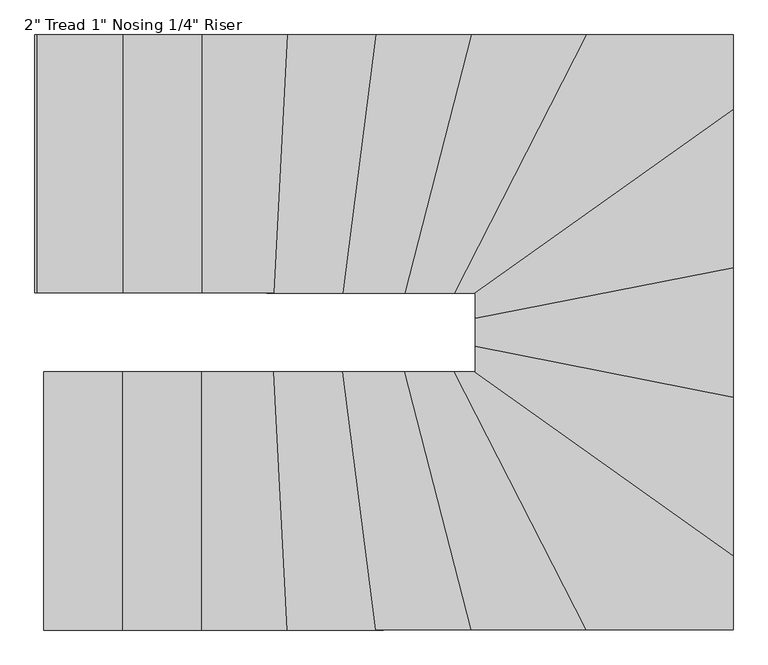
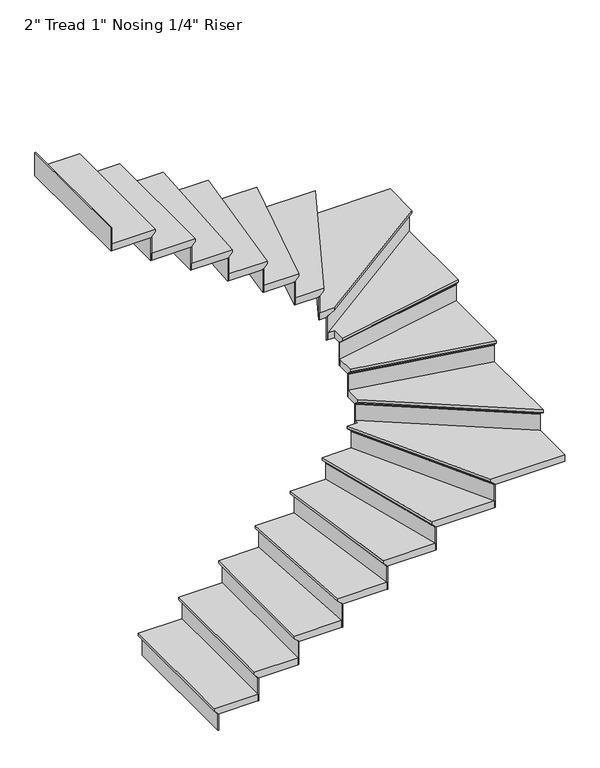
"""IFC4 building model written with IfcOpenShell, lengths in millimetres: stair flight geometry."""

from ifc_helpers import new_model, si_unit, origin, place, context, project, spatial, faceted_brep, source, transform, mapped, element, save


def stair_flight_c0e8b595(model_context):
    return source(origin(), model_context, "Body", "Brep", [
        faceted_brep([(531.7538115, -7565.2090409, 150.2833333), (531.7538115, -7565.2090409, 169.3333333), (531.7538115, -6650.8090409, 169.3333333), (531.7538115, -6650.8090409, 150.2833333), (557.1538115, -7565.2090409, 124.8833333), (557.1538115, -6650.8090409, 124.8833333), (836.5538115, -7565.2090409, 169.3333333), (836.5538115, -6650.8090409, 169.3333333), (557.1538115, -6650.8090409, 118.5333333), (836.5538115, -6650.8090409, 118.5333333), (836.5538115, -7565.2090409, 118.5333333), (557.1538115, -7565.2090409, 118.5333333)], [[[0, 1, 2, 3]], [[4, 0, 3, 5]], [[2, 1, 6, 7]], [[8, 9, 10, 11]], [[2, 7, 9, 8, 5, 3]], [[8, 11, 4, 5]], [[6, 1, 0, 4, 11, 10]], [[7, 6, 10, 9]]]),
        faceted_brep([(557.1538115, -7565.2090409, 118.5333333), (557.1538115, -7565.2090409, 0.0), (563.5038115, -7565.2090409, 0.0), (563.5038115, -7565.2090409, 118.5333333), (557.1538115, -6650.8090409, 118.5333333), (563.5038115, -6650.8090409, 118.5333333), (563.5038115, -6650.8090409, 0.0), (557.1538115, -6650.8090409, 0.0)], [[[0, 1, 2, 3]], [[4, 5, 6, 7]], [[1, 0, 4, 7]], [[2, 1, 7, 6]], [[3, 2, 6, 5]], [[0, 3, 5, 4]]]),
        faceted_brep([(836.5538115, -7565.2090409, 287.8666667), (836.5538115, -7565.2090409, 118.5333333), (842.9038115, -7565.2090409, 118.5333333), (842.9038115, -7565.2090409, 287.8666667), (836.5538115, -6650.8090409, 287.8666667), (842.9038115, -6650.8090409, 287.8666667), (842.9038115, -6650.8090409, 118.5333333), (836.5538115, -6650.8090409, 118.5333333)], [[[0, 1, 2, 3]], [[4, 5, 6, 7]], [[1, 0, 4, 7]], [[2, 1, 7, 6]], [[3, 2, 6, 5]], [[0, 3, 5, 4]]]),
        faceted_brep([(811.1538115, -6650.8090409, 338.6666667), (811.1538115, -7565.2090409, 338.6666667), (1115.9538115, -7565.2090409, 338.6666667), (1115.9538115, -6650.8090409, 338.6666667), (836.5538115, -6650.8090409, 287.8666667), (1115.9538115, -6650.8090409, 287.8666667), (1115.9538115, -7565.2090409, 287.8666667), (836.5538115, -7565.2090409, 287.8666667), (836.5538115, -6650.8090409, 294.2166667), (811.1538115, -6650.8090409, 319.6166667), (836.5538115, -7565.2090409, 294.2166667), (811.1538115, -7565.2090409, 319.6166667)], [[[0, 1, 2, 3]], [[4, 5, 6, 7]], [[0, 3, 5, 4, 8, 9]], [[4, 7, 10, 8]], [[2, 1, 11, 10, 7, 6]], [[3, 2, 6, 5]], [[11, 1, 0, 9]], [[10, 11, 9, 8]]]),
        faceted_brep([(1115.9538115, -7565.2090409, 457.2), (1115.9538115, -7565.2090409, 287.8666667), (1122.3038115, -7565.2090409, 287.8666667), (1122.3038115, -7565.2090409, 457.2), (1115.9538115, -6650.8090409, 457.2), (1122.3038115, -6650.8090409, 457.2), (1122.3038115, -6650.8090409, 287.8666667), (1115.9538115, -6650.8090409, 287.8666667)], [[[0, 1, 2, 3]], [[4, 5, 6, 7]], [[1, 0, 4, 7]], [[2, 1, 7, 6]], [[3, 2, 6, 5]], [[0, 3, 5, 4]]]),
        faceted_brep([(1090.5538115, -6650.8090409, 508.0), (1090.5538115, -7565.2090409, 508.0), (1419.1552434, -7565.2090409, 508.0), (1371.620973, -6650.8090409, 508.0), (1115.9538115, -6650.8090409, 457.2), (1371.620973, -6650.8090409, 457.2), (1419.1552434, -7565.2090409, 457.2), (1115.9538115, -7565.2090409, 457.2), (1115.9538115, -6650.8090409, 463.55), (1090.5538115, -6650.8090409, 488.95), (1115.9538115, -7565.2090409, 463.55), (1090.5538115, -7565.2090409, 488.95)], [[[0, 1, 2, 3]], [[4, 5, 6, 7]], [[0, 3, 5, 4, 8, 9]], [[4, 7, 10, 8]], [[2, 1, 11, 10, 7, 6]], [[3, 2, 6, 5]], [[11, 1, 0, 9]], [[10, 11, 9, 8]]]),
        faceted_brep([(1419.1552434, -7565.2090409, 626.5333333), (1419.1552434, -7565.2090409, 457.2), (1425.5138176, -7565.2090409, 457.2), (1425.5138176, -7565.2090409, 626.5333333), (1371.620973, -6650.8090409, 626.5333333), (1377.9795471, -6650.8090409, 626.5333333), (1377.9795471, -6650.8090409, 457.2), (1371.620973, -6650.8090409, 457.2)], [[[0, 1, 2, 3]], [[4, 5, 6, 7]], [[1, 0, 4, 7]], [[2, 1, 7, 6]], [[3, 2, 6, 5]], [[0, 3, 5, 4]]]),
        faceted_brep([(1346.1866763, -6650.8090409, 677.3333333), (1393.7209467, -7565.2090409, 677.3333333), (1734.1437245, -7565.2090409, 677.3333333), (1615.7876728, -6650.8090409, 677.3333333), (1371.620973, -6650.8090409, 626.5333333), (1615.7876728, -6650.8090409, 626.5333333), (1734.1437245, -7565.2090409, 626.5333333), (1419.1552434, -7565.2090409, 626.5333333), (1371.620973, -6650.8090409, 632.8833333), (1346.1866763, -6650.8090409, 658.2833333), (1419.1552434, -7565.2090409, 632.8833333), (1393.7209467, -7565.2090409, 658.2833333)], [[[0, 1, 2, 3]], [[4, 5, 6, 7]], [[0, 3, 5, 4, 8, 9]], [[4, 7, 10, 8]], [[2, 1, 11, 10, 7, 6]], [[3, 2, 6, 5]], [[11, 1, 0, 9]], [[10, 11, 9, 8]]]),
        faceted_brep([(1734.1437245, -7565.2090409, 795.8666667), (1734.1437245, -7565.2090409, 626.5333333), (1740.5466962, -7565.2090409, 626.5333333), (1740.5466962, -7565.2090409, 795.8666667), (1615.7876728, -6650.8090409, 795.8666667), (1622.1906446, -6650.8090409, 795.8666667), (1622.1906446, -6650.8090409, 626.5333333), (1615.7876728, -6650.8090409, 626.5333333)], [[[0, 1, 2, 3]], [[4, 5, 6, 7]], [[1, 0, 4, 7]], [[2, 1, 7, 6]], [[3, 2, 6, 5]], [[0, 3, 5, 4]]]),
        faceted_brep([(1590.1757857, -6650.8090409, 846.6666667), (1708.5318374, -7565.2090409, 846.6666667), (2072.5453427, -7565.2090409, 846.6666667), (1837.4148953, -6650.8090409, 846.6666667), (1615.7876728, -6650.8090409, 795.8666667), (1837.4148953, -6650.8090409, 795.8666667), (2072.5453427, -7565.2090409, 795.8666667), (1734.1437245, -7565.2090409, 795.8666667), (1615.7876728, -6650.8090409, 802.2166667), (1590.1757857, -6650.8090409, 827.6166667), (1734.1437245, -7565.2090409, 802.2166667), (1708.5318374, -7565.2090409, 827.6166667)], [[[0, 1, 2, 3]], [[4, 5, 6, 7]], [[0, 3, 5, 4, 8, 9]], [[4, 7, 10, 8]], [[2, 1, 11, 10, 7, 6]], [[3, 2, 6, 5]], [[11, 1, 0, 9]], [[10, 11, 9, 8]]]),
        faceted_brep([(2072.5453427, -7565.2090409, 965.2), (2072.5453427, -7565.2090409, 795.8666667), (2079.1019196, -7565.2090409, 795.8666667), (2079.1019196, -7565.2090409, 965.2), (1837.4148953, -6650.8090409, 965.2), (1843.9714722, -6650.8090409, 965.2), (1843.9714722, -6650.8090409, 795.8666667), (1837.4148953, -6650.8090409, 795.8666667)], [[[0, 1, 2, 3]], [[4, 5, 6, 7]], [[1, 0, 4, 7]], [[2, 1, 7, 6]], [[3, 2, 6, 5]], [[0, 3, 5, 4]]]),
        faceted_brep([(1811.1885878, -6650.8090409, 1016.0), (2046.3190352, -7565.2090409, 1016.0), (2482.5861527, -7565.2090409, 1016.0), (2013.7615314, -6650.8090409, 1016.0), (1837.4148953, -6650.8090409, 965.2), (2013.7615314, -6650.8090409, 965.2), (2482.5861527, -7565.2090409, 965.2), (2072.5453427, -7565.2090409, 965.2), (1837.4148953, -6650.8090409, 971.55), (1811.1885878, -6650.8090409, 996.95), (2072.5453427, -7565.2090409, 971.55), (2046.3190352, -7565.2090409, 996.95)], [[[0, 1, 2, 3]], [[4, 5, 6, 7]], [[0, 3, 5, 4, 8, 9]], [[4, 7, 10, 8]], [[2, 1, 11, 10, 7, 6]], [[3, 2, 6, 5]], [[11, 1, 0, 9]], [[10, 11, 9, 8]]]),
        faceted_brep([(2482.5861527, -7565.2090409, 1134.5333333), (2482.5861527, -7565.2090409, 965.2), (2489.7221358, -7565.2090409, 965.2), (2489.7221358, -7565.2090409, 1134.5333333), (2013.7615314, -6650.8090409, 1134.5333333), (2020.8975145, -6650.8090409, 1134.5333333), (2020.8975145, -6650.8090409, 965.2), (2013.7615314, -6650.8090409, 965.2)], [[[0, 1, 2, 3]], [[4, 5, 6, 7]], [[1, 0, 4, 7]], [[2, 1, 7, 6]], [[3, 2, 6, 5]], [[0, 3, 5, 4]]]),
        faceted_brep([(2059.4855034, -6621.253958, 1185.3333333), (2059.4855034, -6650.8090409, 1185.3333333), (1985.2175988, -6650.8090409, 1185.3333333), (2454.0422202, -7565.2090409, 1185.3333333), (2973.8855034, -7565.2090409, 1185.3333333), (2973.8855034, -7271.5279072, 1185.3333333), (2059.4855034, -6650.8090409, 1134.5333333), (2059.4855034, -6621.253958, 1134.5333333), (2973.8855034, -7271.5279072, 1134.5333333), (2973.8855034, -7565.2090409, 1134.5333333), (2482.5861527, -7565.2090409, 1134.5333333), (2013.7615314, -6650.8090409, 1134.5333333), (2013.7615314, -6650.8090409, 1140.8833333), (1985.2175988, -6650.8090409, 1166.2833333), (2482.5861527, -7565.2090409, 1140.8833333), (2454.0422202, -7565.2090409, 1166.2833333)], [[[0, 1, 2, 3, 4, 5]], [[6, 7, 8, 9, 10, 11]], [[1, 0, 7, 6]], [[2, 1, 6, 11, 12, 13]], [[11, 10, 14, 12]], [[4, 3, 15, 14, 10, 9]], [[5, 4, 9, 8]], [[0, 5, 8, 7]], [[15, 3, 2, 13]], [[14, 15, 13, 12]]]),
        faceted_brep([(2973.8855034, -7271.5279072, 1303.8666667), (2973.8855034, -7271.5279072, 1134.5333333), (2973.8855034, -7263.7359324, 1134.5333333), (2973.8855034, -7263.7359324, 1303.8666667), (2059.4855034, -6621.253958, 1303.8666667), (2059.4855034, -6613.4619832, 1303.8666667), (2059.4855034, -6613.4619832, 1134.5333333), (2059.4855034, -6621.253958, 1134.5333333)], [[[0, 1, 2, 3]], [[4, 5, 6, 7]], [[1, 0, 4, 7]], [[2, 1, 7, 6]], [[3, 2, 6, 5]], [[0, 3, 5, 4]]]),
        faceted_brep([(2059.4855034, -6652.4218572, 1354.6666667), (2973.8855034, -7302.6958063, 1354.6666667), (2973.8855034, -6715.0407273, 1354.6666667), (2059.4855034, -6534.7998709, 1354.6666667), (2059.4855034, -6621.253958, 1303.8666667), (2059.4855034, -6534.7998709, 1303.8666667), (2973.8855034, -6715.0407273, 1303.8666667), (2973.8855034, -7271.5279072, 1303.8666667), (2059.4855034, -6621.253958, 1310.2166667), (2059.4855034, -6652.4218572, 1335.6166667), (2973.8855034, -7271.5279072, 1310.2166667), (2973.8855034, -7302.6958063, 1335.6166667)], [[[0, 1, 2, 3]], [[4, 5, 6, 7]], [[0, 3, 5, 4, 8, 9]], [[4, 7, 10, 8]], [[3, 2, 6, 5]], [[11, 1, 0, 9]], [[10, 11, 9, 8]], [[2, 1, 11, 10, 7, 6]]]),
        faceted_brep([(2973.8855034, -6715.0407273, 1473.2), (2973.8855034, -6715.0407273, 1303.8666667), (2973.8855034, -6708.5685418, 1303.8666667), (2973.8855034, -6708.5685418, 1473.2), (2059.4855034, -6534.7998709, 1473.2), (2059.4855034, -6528.3276855, 1473.2), (2059.4855034, -6528.3276855, 1303.8666667), (2059.4855034, -6534.7998709, 1303.8666667)], [[[0, 1, 2, 3]], [[4, 5, 6, 7]], [[1, 0, 4, 7]], [[2, 1, 7, 6]], [[3, 2, 6, 5]], [[0, 3, 5, 4]]]),
        faceted_brep([(2059.4855034, -6560.6886127, 1524.0), (2973.8855034, -6740.929469, 1524.0), (2973.8855034, -6255.3998709, 1524.0), (2059.4855034, -6435.6407273, 1524.0), (2059.4855034, -6534.7998709, 1473.2), (2059.4855034, -6435.6407273, 1473.2), (2973.8855034, -6255.3998709, 1473.2), (2973.8855034, -6715.0407273, 1473.2), (2059.4855034, -6534.7998709, 1479.55), (2059.4855034, -6560.6886127, 1504.95), (2973.8855034, -6715.0407273, 1479.55), (2973.8855034, -6740.929469, 1504.95)], [[[0, 1, 2, 3]], [[4, 5, 6, 7]], [[0, 3, 5, 4, 8, 9]], [[4, 7, 10, 8]], [[2, 1, 11, 10, 7, 6]], [[3, 2, 6, 5]], [[11, 1, 0, 9]], [[10, 11, 9, 8]]]),
        faceted_brep([(2973.8855034, -6255.3998709, 1642.5333333), (2973.8855034, -6255.3998709, 1473.2), (2973.8855034, -6248.9276855, 1473.2), (2973.8855034, -6248.9276855, 1642.5333333), (2059.4855034, -6435.6407273, 1642.5333333), (2059.4855034, -6429.1685418, 1642.5333333), (2059.4855034, -6429.1685418, 1473.2), (2059.4855034, -6435.6407273, 1473.2)], [[[0, 1, 2, 3]], [[4, 5, 6, 7]], [[1, 0, 4, 7]], [[2, 1, 7, 6]], [[3, 2, 6, 5]], [[0, 3, 5, 4]]]),
        faceted_brep([(2013.3900289, -6371.4090409, 1693.3333333), (2059.4855034, -6371.4090409, 1693.3333333), (2059.4855034, -6461.529469, 1693.3333333), (2973.8855034, -6281.2886127, 1693.3333333), (2973.8855034, -5688.3543762, 1693.3333333), (2059.4855034, -6371.4090409, 1642.5333333), (2013.3900289, -6371.4090409, 1642.5333333), (2973.8855034, -5688.3543762, 1642.5333333), (2973.8855034, -6255.3998709, 1642.5333333), (2059.4855034, -6435.6407273, 1642.5333333), (2973.8855034, -6255.3998709, 1648.8833333), (2059.4855034, -6435.6407273, 1648.8833333), (2973.8855034, -6281.2886127, 1674.2833333), (2059.4855034, -6461.529469, 1674.2833333)], [[[0, 1, 2, 3, 4]], [[5, 6, 7, 8, 9]], [[1, 0, 6, 5]], [[9, 8, 10, 11]], [[4, 3, 12, 10, 8, 7]], [[0, 4, 7, 6]], [[12, 3, 2, 13]], [[10, 12, 13, 11]], [[2, 1, 5, 9, 11, 13]]]),
        faceted_brep([(2973.8855034, -5688.3543762, 1811.8666667), (2973.8855034, -5688.3543762, 1642.5333333), (2973.8855034, -5680.5624014, 1642.5333333), (2973.8855034, -5680.5624014, 1811.8666667), (2013.3900289, -6371.4090409, 1811.8666667), (2002.4331364, -6371.4090409, 1811.8666667), (2002.4331364, -6371.4090409, 1642.5333333), (2013.3900289, -6371.4090409, 1642.5333333)], [[[0, 1, 2, 3]], [[4, 5, 6, 7]], [[1, 0, 4, 7]], [[2, 1, 7, 6]], [[3, 2, 6, 5]], [[0, 3, 5, 4]]]),
        faceted_brep([(2057.2175988, -6371.4090409, 1862.6666667), (2973.8855034, -5719.5222754, 1862.6666667), (2973.8855034, -5457.0090409, 1862.6666667), (2425.4982876, -5457.0090409, 1862.6666667), (1956.6736663, -6371.4090409, 1862.6666667), (2013.3900289, -6371.4090409, 1811.8666667), (1956.6736663, -6371.4090409, 1811.8666667), (2425.4982876, -5457.0090409, 1811.8666667), (2973.8855034, -5457.0090409, 1811.8666667), (2973.8855034, -5688.3543762, 1811.8666667), (2013.3900289, -6371.4090409, 1818.2166667), (2057.2175988, -6371.4090409, 1843.6166667), (2973.8855034, -5688.3543762, 1818.2166667), (2973.8855034, -5719.5222754, 1843.6166667)], [[[0, 1, 2, 3, 4]], [[5, 6, 7, 8, 9]], [[0, 4, 6, 5, 10, 11]], [[5, 9, 12, 10]], [[2, 1, 13, 12, 9, 8]], [[4, 3, 7, 6]], [[13, 1, 0, 11]], [[12, 13, 11, 10]], [[3, 2, 8, 7]]]),
        faceted_brep([(2425.4982876, -5457.0090409, 1981.2), (2425.4982876, -5457.0090409, 1811.8666667), (2418.3623045, -5457.0090409, 1811.8666667), (2418.3623045, -5457.0090409, 1981.2), (1956.6736663, -6371.4090409, 1981.2), (1949.5376832, -6371.4090409, 1981.2), (1949.5376832, -6371.4090409, 1811.8666667), (1956.6736663, -6371.4090409, 1811.8666667)], [[[0, 1, 2, 3]], [[4, 5, 6, 7]], [[1, 0, 4, 7]], [[2, 1, 7, 6]], [[3, 2, 6, 5]], [[0, 3, 5, 4]]]),
        faceted_brep([(1985.2175988, -6371.4090409, 2032.0), (2454.0422202, -5457.0090409, 2032.0), (2020.0927278, -5457.0090409, 2032.0), (1784.9622804, -6371.4090409, 2032.0), (1956.6736663, -6371.4090409, 1981.2), (1784.9622804, -6371.4090409, 1981.2), (2020.0927278, -5457.0090409, 1981.2), (2425.4982876, -5457.0090409, 1981.2), (1956.6736663, -6371.4090409, 1987.55), (1985.2175988, -6371.4090409, 2012.95), (2425.4982876, -5457.0090409, 1987.55), (2454.0422202, -5457.0090409, 2012.95)], [[[0, 1, 2, 3]], [[4, 5, 6, 7]], [[0, 3, 5, 4, 8, 9]], [[4, 7, 10, 8]], [[2, 1, 11, 10, 7, 6]], [[3, 2, 6, 5]], [[11, 1, 0, 9]], [[10, 11, 9, 8]]]),
        faceted_brep([(2020.0927278, -5457.0090409, 2150.5333333), (2020.0927278, -5457.0090409, 1981.2), (2013.5361509, -5457.0090409, 1981.2), (2013.5361509, -5457.0090409, 2150.5333333), (1784.9622804, -6371.4090409, 2150.5333333), (1778.4057035, -6371.4090409, 2150.5333333), (1778.4057035, -6371.4090409, 1981.2), (1784.9622804, -6371.4090409, 1981.2)], [[[0, 1, 2, 3]], [[4, 5, 6, 7]], [[1, 0, 4, 7]], [[2, 1, 7, 6]], [[3, 2, 6, 5]], [[0, 3, 5, 4]]]),
        faceted_brep([(1811.1885878, -6371.4090409, 2201.3333333), (2046.3190352, -5457.0090409, 2201.3333333), (1682.9199502, -5457.0090409, 2201.3333333), (1564.5638986, -6371.4090409, 2201.3333333), (1784.9622804, -6371.4090409, 2150.5333333), (1564.5638986, -6371.4090409, 2150.5333333), (1682.9199502, -5457.0090409, 2150.5333333), (2020.0927278, -5457.0090409, 2150.5333333), (1784.9622804, -6371.4090409, 2156.8833333), (1811.1885878, -6371.4090409, 2182.2833333), (2020.0927278, -5457.0090409, 2156.8833333), (2046.3190352, -5457.0090409, 2182.2833333)], [[[0, 1, 2, 3]], [[4, 5, 6, 7]], [[0, 3, 5, 4, 8, 9]], [[4, 7, 10, 8]], [[2, 1, 11, 10, 7, 6]], [[3, 2, 6, 5]], [[11, 1, 0, 9]], [[10, 11, 9, 8]]]),
        faceted_brep([(1682.9199502, -5457.0090409, 2319.8666667), (1682.9199502, -5457.0090409, 2150.5333333), (1676.5169785, -5457.0090409, 2150.5333333), (1676.5169785, -5457.0090409, 2319.8666667), (1564.5638986, -6371.4090409, 2319.8666667), (1558.1609268, -6371.4090409, 2319.8666667), (1558.1609268, -6371.4090409, 2150.5333333), (1564.5638986, -6371.4090409, 2150.5333333)], [[[0, 1, 2, 3]], [[4, 5, 6, 7]], [[1, 0, 4, 7]], [[2, 1, 7, 6]], [[3, 2, 6, 5]], [[0, 3, 5, 4]]]),
        faceted_brep([(1590.1757857, -6371.4090409, 2370.6666667), (1708.5318374, -5457.0090409, 2370.6666667), (1368.2866501, -5457.0090409, 2370.6666667), (1320.7523797, -6371.4090409, 2370.6666667), (1564.5638986, -6371.4090409, 2319.8666667), (1320.7523797, -6371.4090409, 2319.8666667), (1368.2866501, -5457.0090409, 2319.8666667), (1682.9199502, -5457.0090409, 2319.8666667), (1564.5638986, -6371.4090409, 2326.2166667), (1590.1757857, -6371.4090409, 2351.6166667), (1682.9199502, -5457.0090409, 2326.2166667), (1708.5318374, -5457.0090409, 2351.6166667)], [[[0, 1, 2, 3]], [[4, 5, 6, 7]], [[0, 3, 5, 4, 8, 9]], [[4, 7, 10, 8]], [[2, 1, 11, 10, 7, 6]], [[3, 2, 6, 5]], [[11, 1, 0, 9]], [[10, 11, 9, 8]]]),
        faceted_brep([(1368.2866501, -5457.0090409, 2489.2), (1368.2866501, -5457.0090409, 2319.8666667), (1361.9280759, -5457.0090409, 2319.8666667), (1361.9280759, -5457.0090409, 2489.2), (1320.7523797, -6371.4090409, 2489.2), (1314.3938055, -6371.4090409, 2489.2), (1314.3938055, -6371.4090409, 2319.8666667), (1320.7523797, -6371.4090409, 2319.8666667)], [[[0, 1, 2, 3]], [[4, 5, 6, 7]], [[1, 0, 4, 7]], [[2, 1, 7, 6]], [[3, 2, 6, 5]], [[0, 3, 5, 4]]]),
        faceted_brep([(1346.1866763, -6371.4090409, 2540.0), (1393.7209467, -5457.0090409, 2540.0), (1065.1538115, -5457.0090409, 2540.0), (1065.1538115, -6371.4090409, 2540.0), (1320.7523797, -6371.4090409, 2489.2), (1065.1538115, -6371.4090409, 2489.2), (1065.1538115, -5457.0090409, 2489.2), (1368.2866501, -5457.0090409, 2489.2), (1320.7523797, -6371.4090409, 2495.55), (1346.1866763, -6371.4090409, 2520.95), (1368.2866501, -5457.0090409, 2495.55), (1393.7209467, -5457.0090409, 2520.95)], [[[0, 1, 2, 3]], [[4, 5, 6, 7]], [[0, 3, 5, 4, 8, 9]], [[4, 7, 10, 8]], [[2, 1, 11, 10, 7, 6]], [[3, 2, 6, 5]], [[11, 1, 0, 9]], [[10, 11, 9, 8]]]),
        faceted_brep([(1065.1538115, -5457.0090409, 2658.5333333), (1065.1538115, -5457.0090409, 2489.2), (1058.8038115, -5457.0090409, 2489.2), (1058.8038115, -5457.0090409, 2658.5333333), (1065.1538115, -6371.4090409, 2658.5333333), (1058.8038115, -6371.4090409, 2658.5333333), (1058.8038115, -6371.4090409, 2489.2), (1065.1538115, -6371.4090409, 2489.2)], [[[0, 1, 2, 3]], [[4, 5, 6, 7]], [[1, 0, 4, 7]], [[2, 1, 7, 6]], [[3, 2, 6, 5]], [[0, 3, 5, 4]]]),
        faceted_brep([(1090.5538115, -6371.4090409, 2709.3333333), (1090.5538115, -5457.0090409, 2709.3333333), (785.7538115, -5457.0090409, 2709.3333333), (785.7538115, -6371.4090409, 2709.3333333), (1065.1538115, -6371.4090409, 2658.5333333), (785.7538115, -6371.4090409, 2658.5333333), (785.7538115, -5457.0090409, 2658.5333333), (1065.1538115, -5457.0090409, 2658.5333333), (1065.1538115, -6371.4090409, 2664.8833333), (1090.5538115, -6371.4090409, 2690.2833333), (1065.1538115, -5457.0090409, 2664.8833333), (1090.5538115, -5457.0090409, 2690.2833333)], [[[0, 1, 2, 3]], [[4, 5, 6, 7]], [[0, 3, 5, 4, 8, 9]], [[4, 7, 10, 8]], [[2, 1, 11, 10, 7, 6]], [[3, 2, 6, 5]], [[11, 1, 0, 9]], [[10, 11, 9, 8]]]),
        faceted_brep([(785.7538115, -5457.0090409, 2827.8666667), (785.7538115, -5457.0090409, 2658.5333333), (779.4038115, -5457.0090409, 2658.5333333), (779.4038115, -5457.0090409, 2827.8666667), (785.7538115, -6371.4090409, 2827.8666667), (779.4038115, -6371.4090409, 2827.8666667), (779.4038115, -6371.4090409, 2658.5333333), (785.7538115, -6371.4090409, 2658.5333333)], [[[0, 1, 2, 3]], [[4, 5, 6, 7]], [[1, 0, 4, 7]], [[2, 1, 7, 6]], [[3, 2, 6, 5]], [[0, 3, 5, 4]]]),
        faceted_brep([(506.3538115, -5457.0090409, 2997.2), (506.3538115, -5457.0090409, 2827.8666667), (500.0038115, -5457.0090409, 2827.8666667), (500.0038115, -5457.0090409, 2997.2), (506.3538115, -6371.4090409, 2997.2), (500.0038115, -6371.4090409, 2997.2), (500.0038115, -6371.4090409, 2827.8666667), (506.3538115, -6371.4090409, 2827.8666667)], [[[0, 1, 2, 3]], [[4, 5, 6, 7]], [[1, 0, 4, 7]], [[2, 1, 7, 6]], [[3, 2, 6, 5]], [[0, 3, 5, 4]]]),
        faceted_brep([(811.1538115, -6371.4090409, 2878.6666667), (811.1538115, -5457.0090409, 2878.6666667), (506.3538115, -5457.0090409, 2878.6666667), (506.3538115, -6371.4090409, 2878.6666667), (785.7538115, -6371.4090409, 2827.8666667), (506.3538115, -6371.4090409, 2827.8666667), (506.3538115, -5457.0090409, 2827.8666667), (785.7538115, -5457.0090409, 2827.8666667), (785.7538115, -6371.4090409, 2834.2166667), (811.1538115, -6371.4090409, 2859.6166667), (785.7538115, -5457.0090409, 2834.2166667), (811.1538115, -5457.0090409, 2859.6166667)], [[[0, 1, 2, 3]], [[4, 5, 6, 7]], [[0, 3, 5, 4, 8, 9]], [[4, 7, 10, 8]], [[2, 1, 11, 10, 7, 6]], [[3, 2, 6, 5]], [[11, 1, 0, 9]], [[10, 11, 9, 8]]]),
    ])


if __name__ == "__main__":
    model = new_model("IFC4")
    model_context = context("Model", 3, world=origin())
    ifc_project = project(units=[si_unit("LENGTHUNIT", "METRE", prefix="MILLI")], contexts=[model_context])
    site = spatial("IfcSite", under=ifc_project)
    building = spatial("IfcBuilding", under=site)
    placement = place(None, origin())
    stair_flight_shape = stair_flight_c0e8b595(model_context)
    element("IfcStairFlight", 1, ObjectType="2\" Tread 1\" Nosing 1/4\" Riser", at=placement, inside=building, context=model_context, shape_type="MappedRepresentation", body=[
        mapped(stair_flight_shape, transform((0.0, 0.0, 0.0), x_axis=(1.0, 0.0, 0.0), y_axis=(0.0, 1.0, 0.0), z_axis=(0.0, 0.0, 1.0))),
    ])
    save(model, "model.ifc")
